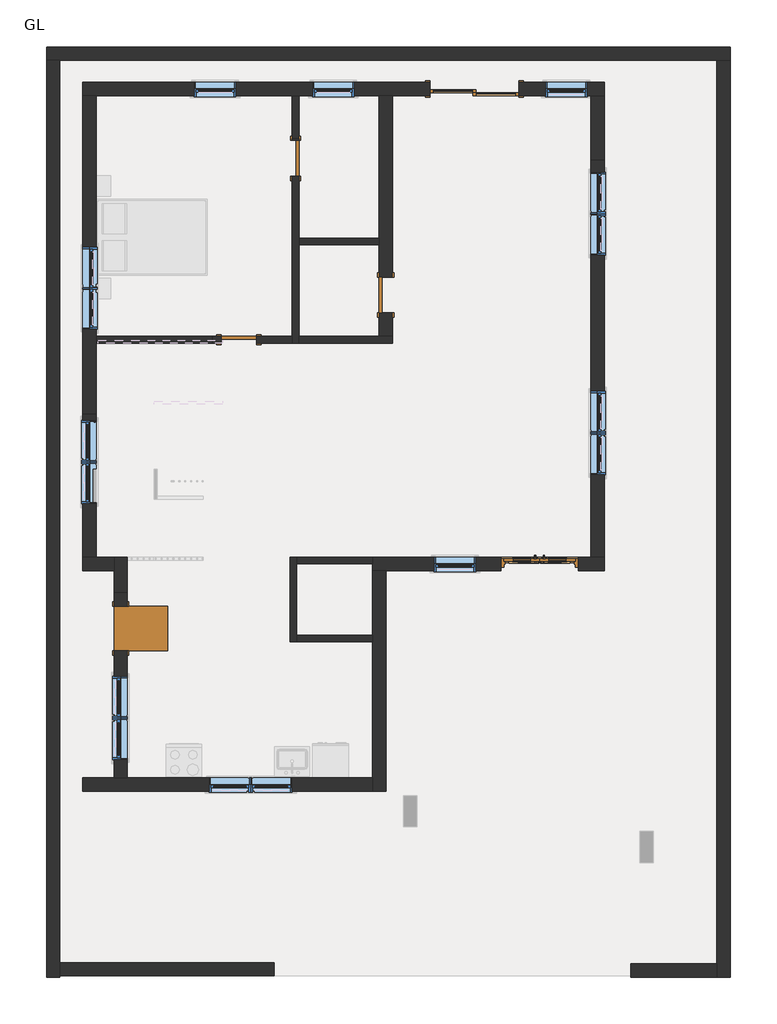
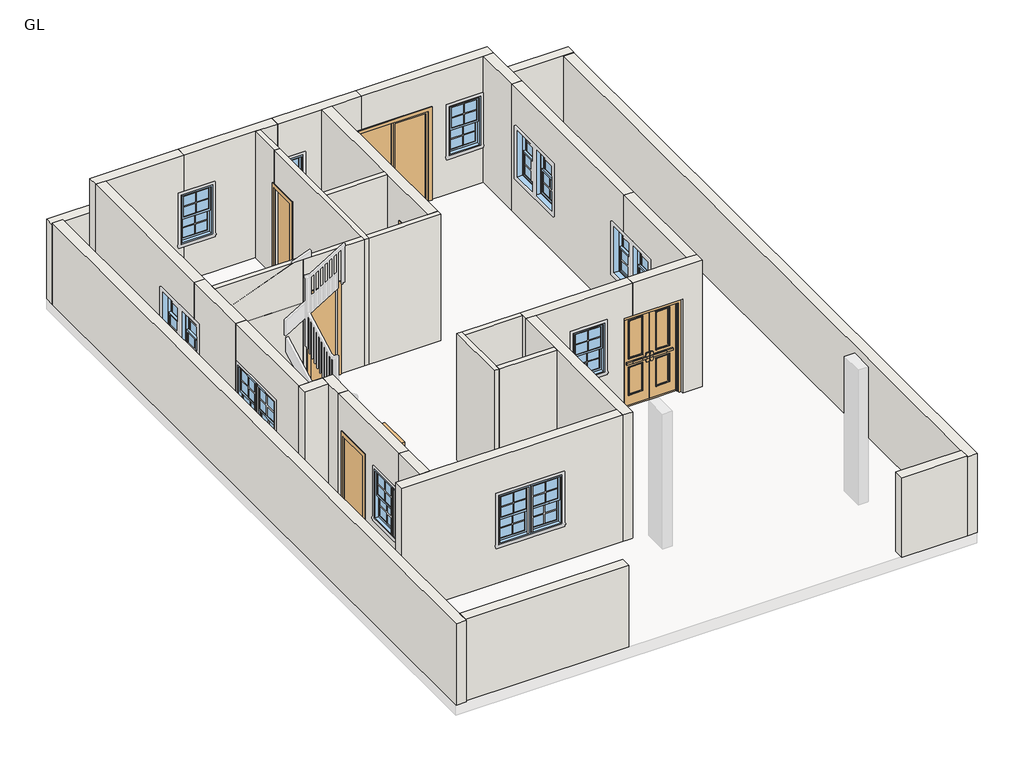
# One storey, part 1 of 3: 33 walls, 16 windows, 6 doors.
"""IFC4 building model written with IfcOpenShell, lengths in millimetres."""

from ifc_helpers import new_model, si_unit, frame, origin, origin_with_axes, place, context, project, spatial, polyline, outline, extrude, faceted_brep, transform, mapped, element, save
from components import door_238c678e, door_exterior_double_two_lite_door_exterior_double_two_lite_a6b01c7a, door_exterior_double_two_lite_door_exterior_double_two_lite_31e28e64, door_exterior_double_two_lite_door_exterior_double_two_lite_4a402bc0, single_flush_2_x_7_f433b8c7, door_0bf9f8da, door_0d3b4037, window_fc4bf0c6

model = new_model("IFC4")

# Units and contexts
model_context = context("Model", 3, world=origin())
ifc_project = project(units=[si_unit("LENGTHUNIT", "METRE", prefix="MILLI")], contexts=[model_context])

# Site, building, storey
site = spatial("IfcSite", under=ifc_project)
building = spatial("IfcBuilding", under=site)
storey = spatial("IfcBuildingStorey", under=building, Name="GL", Elevation=0.0)

# Doors
placement = place(None, origin())
door_shape = door_238c678e(model_context)
element("IfcDoor", 1, ObjectType="Door-Double-Sliding : 60\" x 84\"", at=placement, inside=storey, context=model_context, shape_type="MappedRepresentation", body=[
    mapped(door_shape, transform((-15781.8310804, 12791.3223147, 0.0), x_axis=(-1.0, 0.0, 0.0), y_axis=(0.0, -1.0, 0.0), z_axis=(0.0, 0.0, 1.0))),
])
door_exterior_double_two_lite_door_exterior_double_two_lite_shape = door_exterior_double_two_lite_door_exterior_double_two_lite_a6b01c7a(model_context)
door_exterior_double_two_lite_door_exterior_double_two_lite_2_shape = door_exterior_double_two_lite_door_exterior_double_two_lite_31e28e64(model_context)
door_exterior_double_two_lite_door_exterior_double_two_lite_3_shape = door_exterior_double_two_lite_door_exterior_double_two_lite_4a402bc0(model_context)
element("IfcDoor", 2, ObjectType="Door-Exterior-Double-Two_Lite : Door-Exterior-Double-Two_Lite", at=placement, inside=storey, context=model_context, shape_type="MappedRepresentation", body=[
    mapped(door_exterior_double_two_lite_door_exterior_double_two_lite_shape, transform((-14665.6751671, 4542.6723646, 0.0), x_axis=(1.0, 0.0, 0.0), y_axis=(0.0, 1.0, 0.0), z_axis=(0.0, 0.0, 1.0))),
    mapped(door_exterior_double_two_lite_door_exterior_double_two_lite_2_shape, transform((-14665.6751671, 4542.6723646, 0.0), x_axis=(1.0, 0.0, 0.0), y_axis=(0.0, 1.0, 0.0), z_axis=(0.0, 0.0, 1.0))),
    mapped(door_exterior_double_two_lite_door_exterior_double_two_lite_3_shape, transform((-14665.6751671, 4542.6723646, 0.0), x_axis=(1.0, 0.0, 0.0), y_axis=(0.0, 1.0, 0.0), z_axis=(0.0, 0.0, 1.0))),
])
single_flush_2_x_7_shape = single_flush_2_x_7_f433b8c7(model_context)
element("IfcDoor", 3, ObjectType="Single-Flush : 2' x 7'", at=placement, inside=storey, context=model_context, shape_type="MappedRepresentation", body=[
    mapped(single_flush_2_x_7_shape, transform((-21828.4750314, 3444.1223646, 0.0), x_axis=(0.0, 1.0, 0.0), y_axis=(-1.0, 0.0, 0.0), z_axis=(0.0, 0.0, 1.0))),
])
door_2_shape = door_0bf9f8da(model_context)
element("IfcDoor", 4, ObjectType="Single-Flush : 24\" x 84\"", at=placement, inside=storey, context=model_context, shape_type="MappedRepresentation", body=[
    mapped(door_2_shape, transform((-18837.6250314, 11478.1423646, 0.0), x_axis=(0.0, 1.0, 0.0), y_axis=(-1.0, 0.0, 0.0), z_axis=(0.0, 0.0, 1.0))),
])
element("IfcDoor", 5, ObjectType="Single-Flush : 24\" x 84\"", at=placement, inside=storey, context=model_context, shape_type="MappedRepresentation", body=[
    mapped(door_2_shape, transform((-19809.1750314, 8378.0723646, 0.0), x_axis=(-1.0, 0.0, 0.0), y_axis=(0.0, -1.0, 0.0), z_axis=(0.0, 0.0, 1.0))),
])
door_3_shape = door_0d3b4037(model_context)
element("IfcDoor", 6, ObjectType="Single-Flush : 24\" x 84\"", at=placement, inside=storey, context=model_context, shape_type="MappedRepresentation", body=[
    mapped(door_3_shape, transform((-17294.5750314, 9140.0723646, 0.0), x_axis=(0.0, 1.0, 0.0), y_axis=(-1.0, 0.0, 0.0), z_axis=(0.0, 0.0, 1.0))),
])

# Walls
element("IfcWall", 7, ObjectType="Generic - 4.5\"", at=placement, inside=storey, context=model_context, shape_type="SweptSolid", body=[
    extrude(outline(polyline([(-18894.7750314, 11808.3423646), (-18894.7750314, 12550.0223147), (-18780.4750314, 12550.0223147), (-18780.4750314, 11808.3423646), (-18894.7750314, 11808.3423646)])), origin_with_axes(), (0.0, 0.0, 1.0), 2997.2),
])
element("IfcWall", 8, ObjectType="Generic - 4.5\"", at=placement, inside=storey, context=model_context, shape_type="Brep", body=[
    faceted_brep([(-18894.7750314, 11808.3423646, 0.0), (-18894.7750314, 11782.9423646, 0.0), (-18894.7750314, 11782.9423646, 2133.6), (-18894.7750314, 11173.3423646, 2133.6), (-18894.7750314, 11173.3423646, 0.0), (-18894.7750314, 8435.2223646, 0.0), (-18894.7750314, 8320.9223646, 0.0), (-18894.7750314, 8320.9223646, 2997.2), (-18894.7750314, 8435.2223646, 2997.2), (-18894.7750314, 11808.3423646, 2997.2), (-18780.4750314, 11782.9423646, 2133.6), (-18780.4750314, 11782.9423646, 0.0), (-18780.4750314, 11808.3423646, 0.0), (-18780.4750314, 11808.3423646, 2997.2), (-18780.4750314, 10111.6223646, 2997.2), (-18780.4750314, 9997.3223646, 2997.2), (-18780.4750314, 8435.2223646, 2997.2), (-18780.4750314, 8320.9223646, 2997.2), (-18780.4750314, 8320.9223646, 0.0), (-18780.4750314, 8435.2223646, 0.0), (-18780.4750314, 9997.3223646, 0.0), (-18780.4750314, 10111.6223646, 0.0), (-18780.4750314, 11173.3423646, 0.0), (-18780.4750314, 11173.3423646, 2133.6)], [[[0, 1, 2, 3, 4, 5, 6, 7, 8, 9]], [[10, 11, 12, 13, 14, 15, 16, 17, 18, 19, 20, 21, 22, 23]], [[12, 11, 1, 0]], [[22, 21, 20, 19, 18, 6, 5, 4]], [[0, 9, 13, 12]], [[7, 6, 18, 17]], [[2, 1, 11, 10]], [[3, 2, 10, 23]], [[4, 3, 23, 22]], [[9, 8, 7, 17, 16, 15, 14, 13]]]),
])
element("IfcWall", 9, ObjectType="Generic - 4.5\"", at=placement, inside=storey, context=model_context, shape_type="Brep", body=[
    faceted_brep([(-18780.4750314, 8320.9223646, 0.0), (-17180.2750314, 8320.9223646, 0.0), (-17180.2750314, 8320.9223646, 2997.2), (-18780.4750314, 8320.9223646, 2997.2), (-18780.4750314, 8435.2223646, 0.0), (-18780.4750314, 8435.2223646, 2997.2), (-17408.8750314, 8435.2223646, 2997.2), (-17180.2750314, 8435.2223646, 2997.2), (-17180.2750314, 8435.2223646, 0.0), (-17408.8750314, 8435.2223646, 0.0)], [[[0, 1, 2, 3]], [[4, 5, 6, 7, 8, 9]], [[1, 0, 4, 9, 8]], [[0, 3, 5, 4]], [[2, 1, 8, 7]], [[3, 2, 7, 6, 5]]]),
])
element("IfcWall", 10, ObjectType="Generic - 4.5\"", at=placement, inside=storey, context=model_context, shape_type="SweptSolid", body=[
    extrude(outline(polyline([(0.0, -20266.3750314), (0.0, -20113.9750314), (2133.6, -20113.9750314), (2133.6, -19504.3750314), (0.0, -19504.3750314), (0.0, -18894.7750314), (2997.2, -18894.7750314), (2997.2, -20266.3750314), (0.0, -20266.3750314)])), frame((0.0, 8320.9223646, 0.0), z_axis=(0.0, 1.0, 0.0), x_axis=(0.0, 0.0, 1.0)), (0.0, 0.0, 1.0), 114.3),
])
element("IfcWall", 11, ObjectType="Generic - 4.5\"", at=placement, inside=storey, context=model_context, shape_type="SweptSolid", body=[
    extrude(outline(polyline([(-20266.3750314, 8320.9223646), (-22247.5752061, 8320.9223646), (-22247.5752061, 8435.2223646), (-20266.3750314, 8435.2223646), (-20266.3750314, 8320.9223646)])), origin_with_axes(), (0.0, 0.0, 1.0), 2997.2),
])
element("IfcWall", 12, ObjectType="Generic - 4.5\"", at=placement, inside=storey, context=model_context, shape_type="SweptSolid", body=[
    extrude(outline(polyline([(-17408.8750314, 9997.3223646), (-18780.4750314, 9997.3223646), (-18780.4750314, 10111.6223646), (-17408.8750314, 10111.6223646), (-17408.8750314, 9997.3223646)])), origin_with_axes(), (0.0, 0.0, 1.0), 2997.2),
])
element("IfcWall", 13, ObjectType="Generic - 4.5\"", at=placement, inside=storey, context=model_context, shape_type="Brep", body=[
    faceted_brep([(-18932.8750314, 4663.3223646, 0.0), (-18932.8750314, 3215.5223646, 0.0), (-18932.8750314, 3215.5223646, 2997.2), (-18932.8750314, 4663.3223646, 2997.2), (-18818.5750314, 4663.3223646, 0.0), (-18818.5750314, 4663.3223646, 2997.2), (-18818.5750314, 4549.0223646, 2997.2), (-18818.5750314, 3329.8223646, 2997.2), (-18818.5750314, 3215.5223646, 2997.2), (-18818.5750314, 3215.5223646, 0.0), (-18818.5750314, 3329.8223646, 0.0), (-18818.5750314, 4549.0223646, 0.0)], [[[0, 1, 2, 3]], [[4, 5, 6, 7, 8, 9, 10, 11]], [[1, 0, 4, 11, 10, 9]], [[2, 1, 9, 8]], [[0, 3, 5, 4]], [[3, 2, 8, 7, 6, 5]]]),
])
element("IfcWall", 14, ObjectType="Generic - 4.5\"", at=placement, inside=storey, context=model_context, shape_type="SweptSolid", body=[
    extrude(outline(polyline([(-17523.1750314, 3215.5223646), (-18818.5750314, 3215.5223646), (-18818.5750314, 3329.8223646), (-17523.1750314, 3329.8223646), (-17523.1750314, 3215.5223646)])), origin_with_axes(), (0.0, 0.0, 1.0), 2997.2),
])
element("IfcWall", 15, ObjectType="Generic - 4.5\"", at=placement, inside=storey, context=model_context, shape_type="SweptSolid", body=[
    extrude(outline(polyline([(-17523.1750314, 4549.0223646), (-18818.5750314, 4549.0223646), (-18818.5750314, 4663.3223646), (-17523.1750314, 4663.3223646), (-17523.1750314, 4549.0223646)])), origin_with_axes(), (0.0, 0.0, 1.0), 2997.2),
])
element("IfcWall", 16, ObjectType="Generic - 9\" 2", at=placement, inside=storey, context=model_context, shape_type="Brep", body=[
    faceted_brep([(-11408.7437595, 13378.6077942, 0.0), (-23096.6616791, 13378.6077942, 0.0), (-23096.6616791, 13378.6077942, 1886.4124862), (-11408.7437595, 13378.6077942, 1886.4124862), (-11408.7437595, 13150.0077942, 0.0), (-11408.7437595, 13150.0077942, 1876.4849166), (-11408.7437595, 13150.0077942, 1886.4124862), (-23096.6616791, 13150.0077942, 1886.4124862), (-23096.6616791, 13150.0077942, 0.0), (-22868.0616791, 13150.0077942, 0.0), (-11637.3437595, 13150.0077942, 0.0)], [[[0, 1, 2, 3]], [[4, 5, 6, 7, 8, 9, 10]], [[1, 0, 4, 10, 9, 8]], [[3, 2, 7, 6]], [[2, 1, 8, 7]], [[0, 3, 6, 5, 4]]]),
])
element("IfcWall", 17, ObjectType="Generic - 9\" 2", at=placement, inside=storey, context=model_context, shape_type="Brep", body=[
    faceted_brep([(-23096.6616791, 13150.0077942, 0.0), (-23096.6616791, -2518.5276354, 0.0), (-23096.6616791, -2518.5276354, 1930.400068), (-23096.6616791, 13150.0077942, 1930.400068), (-23096.6616791, 13150.0077942, 1886.4124862), (-22868.0616791, 13150.0077942, 0.0), (-22868.0616791, 13150.0077942, 1930.400068), (-22868.0616791, -2518.5276354, 1930.400068), (-22868.0616791, -2518.5276354, 0.0)], [[[0, 1, 2, 3, 4]], [[5, 6, 7, 8]], [[1, 0, 5, 8]], [[2, 1, 8, 7]], [[3, 2, 7, 6]], [[0, 4, 3, 6, 5]]]),
])
element("IfcWall", 18, ObjectType="Generic - 9\" 2", at=placement, inside=storey, context=model_context, shape_type="SweptSolid", body=[
    extrude(outline(polyline([(-19208.5067292, -2492.7076157), (-22866.1067292, -2492.7076157), (-22866.1067292, -2264.1076157), (-19208.5067292, -2264.1076157), (-19208.5067292, -2492.7076157)])), origin_with_axes(), (0.0, 0.0, 1.0), 1937.5226212),
])
element("IfcWall", 19, ObjectType="Generic - 9\" 2", at=placement, inside=storey, context=model_context, shape_type="Brep", body=[
    faceted_brep([(-11637.3437595, 13150.0077942, 0.0), (-11637.3437595, -2286.8422058, 0.0), (-11637.3437595, -2515.4422058, 0.0), (-11637.3437595, -2515.4422058, 1876.4849166), (-11637.3437595, 13150.0077942, 1876.4849166), (-11408.7437595, 13150.0077942, 0.0), (-11408.7437595, 13150.0077942, 1876.4849166), (-11408.7437595, -2515.4422058, 1876.4849166), (-11408.7437595, -2515.4422058, 0.0)], [[[0, 1, 2, 3, 4]], [[5, 6, 7, 8]], [[2, 1, 0, 5, 8]], [[4, 3, 7, 6]], [[0, 4, 6, 5]], [[3, 2, 8, 7]]]),
])
element("IfcWall", 20, ObjectType="Generic - 9\" 2", at=placement, inside=storey, context=model_context, shape_type="Brep", body=[
    faceted_brep([(-11637.3437595, -2286.8422058, 0.0), (-13103.5750314, -2286.8422058, 0.0), (-13103.5750314, -2286.8422058, 1892.5418489), (-11637.3437595, -2286.8422058, 1892.5418489), (-11637.3437595, -2515.4422058, 0.0), (-11637.3437595, -2515.4422058, 1876.4849166), (-11637.3437595, -2515.4422058, 1892.5418489), (-13103.5750314, -2515.4422058, 1892.5418489), (-13103.5750314, -2515.4422058, 0.0)], [[[0, 1, 2, 3]], [[4, 5, 6, 7, 8]], [[1, 0, 4, 8]], [[2, 1, 8, 7]], [[3, 2, 7, 6]], [[0, 3, 6, 5, 4]]]),
])
element("IfcWall", 21, ObjectType="Generic -9\"Brick 2", at=placement, inside=storey, context=model_context, shape_type="Brep", body=[
    faceted_brep([(-22476.1750314, 12550.0223646, 0.0), (-22247.5750314, 12550.0223646, 0.0), (-20494.9750314, 12550.0223646, 0.0), (-20494.9750314, 12550.0223646, 914.4), (-20571.1750314, 12550.0223646, 914.4), (-20571.1750314, 12550.0223646, 2082.8), (-20494.9750314, 12550.0223646, 2082.8), (-20494.9750314, 12550.0223646, 2997.2), (-22247.5750314, 12550.0223646, 2997.2), (-22476.1752061, 12550.0223646, 2997.2), (-20494.9750314, 12778.6223646, 0.0), (-22476.1750314, 12778.6223646, 0.0), (-22476.1750314, 12778.6223646, 2997.2), (-20494.9750314, 12778.6223646, 2997.2), (-20494.9750314, 12778.6223646, 2082.8), (-20571.1750314, 12778.6223646, 2082.8), (-20571.1750314, 12778.6223646, 914.4), (-20494.9750314, 12778.6223646, 914.4)], [[[0, 1, 2, 3, 4, 5, 6, 7, 8, 9]], [[10, 11, 12, 13, 14, 15, 16, 17]], [[2, 1, 0, 11, 10]], [[2, 10, 17, 3]], [[13, 7, 6, 14]], [[0, 9, 12, 11]], [[16, 4, 3, 17]], [[4, 16, 15, 5]], [[5, 15, 14, 6]], [[9, 8, 7, 13, 12]]]),
])
element("IfcWall", 22, ObjectType="Generic -9\"Brick 2", at=placement, inside=storey, context=model_context, shape_type="Brep", body=[
    faceted_brep([(-20494.9750314, 12550.0223147, 0.0), (-18894.7750314, 12550.0223147, 0.0), (-18780.4750314, 12550.0223147, 0.0), (-18397.0494379, 12550.0223147, 0.0), (-18397.0494379, 12550.0223147, 914.4), (-18549.4494379, 12550.0223147, 914.4), (-18549.4494379, 12550.0223147, 2082.8), (-18397.0494379, 12550.0223147, 2082.8), (-18397.0494379, 12550.0223147, 2997.2), (-18780.4750314, 12550.0223147, 2997.2), (-18894.7750314, 12550.0223147, 2997.2), (-20494.9750314, 12550.0223147, 2997.2), (-20494.9750314, 12550.0223147, 2082.8), (-19859.9750314, 12550.0223147, 2082.8), (-19859.9750314, 12550.0223147, 914.4), (-20494.9750314, 12550.0223147, 914.4), (-18397.0494379, 12778.6223147, 0.0), (-20494.9750314, 12778.6223147, 0.0), (-20494.9750314, 12778.6223147, 914.4), (-19859.9750314, 12778.6223147, 914.4), (-19859.9750314, 12778.6223147, 2082.8), (-20494.9750314, 12778.6223147, 2082.8), (-20494.9750314, 12778.6223147, 2997.2), (-18397.0494379, 12778.6223147, 2997.2), (-18397.0494379, 12778.6223147, 2082.8), (-18549.4494379, 12778.6223147, 2082.8), (-18549.4494379, 12778.6223147, 914.4), (-18397.0494379, 12778.6223147, 914.4)], [[[0, 1, 2, 3, 4, 5, 6, 7, 8, 9, 10, 11, 12, 13, 14, 15]], [[16, 17, 18, 19, 20, 21, 22, 23, 24, 25, 26, 27]], [[3, 2, 1, 0, 17, 16]], [[3, 16, 27, 4]], [[23, 8, 7, 24]], [[17, 0, 15, 18]], [[12, 11, 22, 21]], [[13, 20, 19, 14]], [[14, 19, 18, 15]], [[20, 13, 12, 21]], [[26, 5, 4, 27]], [[5, 26, 25, 6]], [[6, 25, 24, 7]], [[11, 10, 9, 8, 23, 22]]]),
])
element("IfcWall", 23, ObjectType="Generic -9\"Brick 2", at=placement, inside=storey, context=model_context, shape_type="Brep", body=[
    faceted_brep([(-18397.0494379, 12550.0223147, 914.4), (-18397.0494379, 12550.0223147, 0.0), (-17408.8750314, 12550.0223147, 0.0), (-17180.2750314, 12550.0223147, 0.0), (-16543.8310804, 12550.0223147, 0.0), (-16543.8310804, 12550.0223147, 2133.6), (-16518.4310804, 12550.0223147, 2133.6), (-16518.4310804, 12550.0223147, 2997.2), (-17180.2750314, 12550.0223147, 2997.2), (-17408.8750314, 12550.0223147, 2997.2), (-18397.0494379, 12550.0223147, 2997.2), (-18397.0494379, 12550.0223147, 2082.8), (-17838.2494379, 12550.0223147, 2082.8), (-17838.2494379, 12550.0223147, 914.4), (-18397.0494379, 12778.6223147, 0.0), (-18397.0494379, 12778.6223147, 914.4), (-17838.2494379, 12778.6223147, 914.4), (-17838.2494379, 12778.6223147, 2082.8), (-18397.0494379, 12778.6223147, 2082.8), (-18397.0494379, 12778.6223147, 2997.2), (-16518.4310804, 12778.6223147, 2997.2), (-16518.4310804, 12778.6223147, 2133.6), (-16543.8310804, 12778.6223147, 2133.6), (-16543.8310804, 12778.6223147, 0.0)], [[[0, 1, 2, 3, 4, 5, 6, 7, 8, 9, 10, 11, 12, 13]], [[14, 15, 16, 17, 18, 19, 20, 21, 22, 23]], [[1, 14, 23, 4, 3, 2]], [[20, 7, 6, 21]], [[14, 1, 0, 15]], [[11, 10, 19, 18]], [[12, 17, 16, 13]], [[13, 16, 15, 0]], [[17, 12, 11, 18]], [[22, 5, 4, 23]], [[5, 22, 21, 6]], [[10, 9, 8, 7, 20, 19]]]),
])
element("IfcWall", 24, ObjectType="Generic -9\"Brick 2", at=placement, inside=storey, context=model_context, shape_type="Brep", body=[
    faceted_brep([(-13560.7750314, 12550.0223147, 0.0), (-13560.7750314, 12550.0223147, 2997.2), (-13789.3750314, 12550.0223147, 2997.2), (-16518.4310804, 12550.0223147, 2997.2), (-16518.4310804, 12550.0223147, 2133.6), (-15019.8310804, 12550.0223147, 2133.6), (-15019.8310804, 12550.0223147, 0.0), (-13789.3750314, 12550.0223147, 0.0), (-13852.8750314, 12550.0223147, 2082.8), (-13852.8750314, 12550.0223147, 914.4), (-14564.0750314, 12550.0223147, 914.4), (-14564.0750314, 12550.0223147, 2082.8), (-13560.7750314, 12778.6223147, 2997.2), (-13560.7750314, 12778.6223147, 0.0), (-15019.8310804, 12778.6223147, 0.0), (-15019.8310804, 12778.6223147, 2133.6), (-16518.4310804, 12778.6223147, 2133.6), (-16518.4310804, 12778.6223147, 2997.2), (-13852.8750314, 12778.6223147, 2082.8), (-14564.0750314, 12778.6223147, 2082.8), (-14564.0750314, 12778.6223147, 914.4), (-13852.8750314, 12778.6223147, 914.4)], [[[0, 1, 2, 3, 4, 5, 6, 7], [8, 9, 10, 11]], [[12, 13, 14, 15, 16, 17], [18, 19, 20, 21]], [[13, 0, 7, 6, 14]], [[3, 17, 16, 4]], [[1, 0, 13, 12]], [[9, 8, 18, 21]], [[10, 9, 21, 20]], [[11, 10, 20, 19]], [[8, 11, 19, 18]], [[5, 15, 14, 6]], [[15, 5, 4, 16]], [[3, 2, 1, 12, 17]]]),
])
element("IfcWall", 25, ObjectType="Generic -9\"Brick 2", at=placement, inside=storey, context=model_context, shape_type="SweptSolid", body=[
    extrude(outline(polyline([(-13789.3750314, 11447.1098201), (-13789.3750314, 12550.0223147), (-13560.7750314, 12550.0223147), (-13560.7750314, 11447.1098201), (-13789.3750314, 11447.1098201)])), origin_with_axes(), (0.0, 0.0, 1.0), 2997.2),
])
element("IfcWall", 26, ObjectType="Generic -9\"Brick 2", at=placement, inside=storey, context=model_context, shape_type="SweptSolid", body=[
    extrude(outline(polyline([(11447.1098201, 0.0), (7101.7223647, 0.0), (7101.7223647, 914.4), (7495.4223646, 914.4), (7495.4223646, 2082.8), (7101.7223647, 2082.8), (7101.7223647, 2997.2), (11447.1098201, 2997.2), (11447.1098201, 0.0)]), holes=[polyline([(11243.9098201, 914.4), (11243.9098201, 2082.8), (9821.5098201, 2082.8), (9821.5098201, 914.4), (11243.9098201, 914.4)])]), frame((-13789.3750314, 0.0, 0.0), z_axis=(1.0, 0.0, 0.0), x_axis=(0.0, 1.0, 0.0)), (0.0, 0.0, 1.0), 228.6),
])
element("IfcWall", 27, ObjectType="Generic -9\"Brick 2", at=placement, inside=storey, context=model_context, shape_type="SweptSolid", body=[
    extrude(outline(polyline([(7101.7223647, 0.0), (4663.3223646, 0.0), (4663.3223646, 2997.2), (7101.7223647, 2997.2), (7101.7223647, 2082.8), (6073.0223646, 2082.8), (6073.0223646, 914.4), (7101.7223647, 914.4), (7101.7223647, 0.0)])), frame((-13789.3750314, 0.0, 0.0), z_axis=(1.0, 0.0, 0.0), x_axis=(0.0, 1.0, 0.0)), (0.0, 0.0, 1.0), 228.6),
])
element("IfcWall", 28, ObjectType="Generic -9\"Brick 2", at=placement, inside=storey, context=model_context, shape_type="Brep", body=[
    faceted_brep([(-13560.7750314, 4434.7223646, 0.0), (-13560.7750314, 4434.7223646, 2997.2), (-15122.8751671, 4434.7223646, 2997.2), (-15122.8751671, 4434.7223646, 2235.2), (-14005.2751671, 4434.7223646, 2235.2), (-14005.2751671, 4434.7223646, 0.0), (-13560.7750314, 4663.3223646, 2997.2), (-13560.7750314, 4663.3223646, 0.0), (-13789.3750314, 4663.3223646, 0.0), (-14005.2751671, 4663.3223646, 0.0), (-14005.2751671, 4663.3223646, 2235.2), (-15122.8751671, 4663.3223646, 2235.2), (-15122.8751671, 4663.3223646, 2997.2), (-13789.3750314, 4663.3223646, 2997.2)], [[[0, 1, 2, 3, 4, 5]], [[6, 7, 8, 9, 10, 11, 12, 13]], [[7, 0, 5, 9, 8]], [[2, 12, 11, 3]], [[1, 0, 7, 6]], [[4, 10, 9, 5]], [[10, 4, 3, 11]], [[2, 1, 6, 13, 12]]]),
])
element("IfcWall", 29, ObjectType="Generic -9\"Brick 2", at=placement, inside=storey, context=model_context, shape_type="Brep", body=[
    faceted_brep([(-17523.1750314, 4663.3223722, 0.0), (-17523.1750314, 4663.3223722, 2997.2), (-15122.8751671, 4663.3223722, 2997.2), (-15122.8751671, 4663.3223722, 2235.2), (-15326.0751671, 4663.3223722, 2235.2), (-15326.0751671, 4663.3223722, 0.0), (-15757.8750314, 4663.3223722, 2290.2004923), (-16469.0750314, 4663.3223722, 2290.2004923), (-16469.0750314, 4663.3223722, 1121.8004923), (-15757.8750314, 4663.3223722, 1121.8004923), (-17523.1750314, 4434.7223722, 2997.2), (-17523.1750314, 4434.7223722, 0.0), (-17294.5750314, 4434.7223722, 0.0), (-15326.0751671, 4434.7223722, 0.0), (-15326.0751671, 4434.7223722, 2235.2), (-15122.8751671, 4434.7223722, 2235.2), (-15122.8751671, 4434.7223722, 2997.2), (-17294.5750314, 4434.7223722, 2997.2), (-15757.8750314, 4434.7223722, 2290.2004923), (-15757.8750314, 4434.7223722, 1121.8004923), (-16469.0750314, 4434.7223722, 1121.8004923), (-16469.0750314, 4434.7223722, 2290.2004923), (-17523.1750314, 4549.0223646, 0.0), (-17523.1750314, 4549.0223646, 2997.2)], [[[0, 1, 2, 3, 4, 5], [6, 7, 8, 9]], [[10, 11, 12, 13, 14, 15, 16, 17], [18, 19, 20, 21]], [[11, 22, 0, 5, 13, 12]], [[2, 16, 15, 3]], [[1, 0, 22, 11, 10, 23]], [[14, 4, 3, 15]], [[4, 14, 13, 5]], [[2, 1, 23, 10, 17, 16]], [[19, 18, 6, 9]], [[20, 19, 9, 8]], [[21, 20, 8, 7]], [[18, 21, 7, 6]]]),
])
element("IfcWall", 30, ObjectType="Generic -9\"Brick 2", at=placement, inside=storey, context=model_context, shape_type="Brep", body=[
    faceted_brep([(-17523.1750314, 4434.7223722, 0.0), (-17523.1750314, 3329.8223646, 0.0), (-17523.1750314, 3215.5223646, 0.0), (-17523.1750314, 891.4223646, 0.0), (-17523.1750314, 662.8223646, 0.0), (-17523.1750314, 662.8223646, 2997.2), (-17523.1750314, 891.4223646, 2997.2), (-17523.1750314, 3215.5223646, 2997.2), (-17523.1750314, 3329.8223646, 2997.2), (-17523.1750314, 4434.7223722, 2997.2), (-17294.5750314, 4434.7223722, 0.0), (-17294.5750314, 4434.7223722, 2997.2), (-17294.5750314, 662.8223646, 2997.2), (-17294.5750314, 662.8223646, 0.0)], [[[0, 1, 2, 3, 4, 5, 6, 7, 8, 9]], [[10, 11, 12, 13]], [[4, 3, 2, 1, 0, 10, 13]], [[0, 9, 11, 10]], [[5, 4, 13, 12]], [[9, 8, 7, 6, 5, 12, 11]]]),
])
element("IfcWall", 31, ObjectType="Generic -9\"Brick 2", at=placement, inside=storey, context=model_context, shape_type="Brep", body=[
    faceted_brep([(-17523.1750314, 891.4223646, 0.0), (-21714.1750314, 891.4223646, 0.0), (-21942.7750314, 891.4223646, 0.0), (-22476.1750314, 891.4223646, 0.0), (-22476.1750314, 891.4223646, 2997.2), (-21942.7750314, 891.4223646, 2997.2), (-21714.1750314, 891.4223646, 2997.2), (-17523.1750314, 891.4223646, 2997.2), (-18894.6931686, 891.4223646, 2082.8), (-20317.0931686, 891.4223646, 2082.8), (-20317.0931686, 891.4223646, 914.4), (-18894.6931686, 891.4223646, 914.4), (-22476.1750314, 662.8223646, 0.0), (-17523.1750314, 662.8223646, 0.0), (-17523.1750314, 662.8223646, 2997.2), (-22476.1750314, 662.8223646, 2997.2), (-20317.0931686, 662.8223646, 2082.8), (-18894.6931686, 662.8223646, 2082.8), (-18894.6931686, 662.8223646, 914.4), (-20317.0931686, 662.8223646, 914.4)], [[[0, 1, 2, 3, 4, 5, 6, 7], [8, 9, 10, 11]], [[12, 13, 14, 15], [16, 17, 18, 19]], [[3, 2, 1, 0, 13, 12]], [[4, 3, 12, 15]], [[0, 7, 14, 13]], [[16, 9, 8, 17]], [[18, 11, 10, 19]], [[18, 17, 8, 11]], [[19, 10, 9, 16]], [[7, 6, 5, 4, 15, 14]]]),
])
element("IfcWall", 32, ObjectType="Generic -9\"Brick 2", at=placement, inside=storey, context=model_context, shape_type="SweptSolid", body=[
    extrude(outline(polyline([(1710.5723646, 0.0), (891.4223646, 0.0), (891.4223646, 2997.2), (1710.5723646, 2997.2), (1710.5723646, 2082.8), (1202.5723646, 2082.8), (1202.5723646, 914.4), (1710.5723646, 914.4), (1710.5723646, 0.0)])), frame((-21942.7750314, 0.0, 0.0), z_axis=(1.0, 0.0, 0.0), x_axis=(0.0, 1.0, 0.0)), (0.0, 0.0, 1.0), 228.6),
])
element("IfcWall", 33, ObjectType="Generic -9\"Brick 2", at=placement, inside=storey, context=model_context, shape_type="SweptSolid", body=[
    extrude(outline(polyline([(4053.7223646, 0.0), (3825.1223646, 0.0), (3825.1223646, 2133.6), (3063.1223646, 2133.6), (3063.1223646, 0.0), (1710.5723646, 0.0), (1710.5723646, 914.4), (2624.9723646, 914.4), (2624.9723646, 2082.8), (1710.5723646, 2082.8), (1710.5723646, 2997.2), (4053.7223646, 2997.2), (4053.7223646, 0.0)])), frame((-21942.7750314, 0.0, 0.0), z_axis=(1.0, 0.0, 0.0), x_axis=(0.0, 1.0, 0.0)), (0.0, 0.0, 1.0), 228.6),
])
element("IfcWall", 34, ObjectType="Generic -9\"Brick 2", at=placement, inside=storey, context=model_context, shape_type="Brep", body=[
    faceted_brep([(-21714.1750314, 4053.7223646, 0.0), (-21714.1750314, 4663.3223646, 0.0), (-21714.1750314, 4663.3223646, 2997.2), (-21714.1750314, 4053.7223646, 2997.2), (-21942.7750314, 4053.7223646, 0.0), (-21942.7750314, 4053.7223646, 2997.2), (-21942.7750314, 4434.7223646, 2997.2), (-21942.7750314, 4663.3223646, 2997.2), (-21942.7750314, 4663.3223646, 0.0), (-21942.7750314, 4434.7223646, 0.0)], [[[0, 1, 2, 3]], [[4, 5, 6, 7, 8, 9]], [[1, 0, 4, 9, 8]], [[0, 3, 5, 4]], [[2, 1, 8, 7]], [[3, 2, 7, 6, 5]]]),
])
element("IfcWall", 35, ObjectType="Generic -9\"Brick 2", at=placement, inside=storey, context=model_context, shape_type="SweptSolid", body=[
    extrude(outline(polyline([(12550.0223646, 0.0), (8710.539033, 0.0), (8710.539033, 914.4), (9955.139033, 914.4), (9955.139033, 2082.8), (8710.539033, 2082.8), (8710.539033, 2997.2), (12550.0223646, 2997.2), (12550.0223646, 0.0)])), frame((-22476.1750314, 0.0, 0.0), z_axis=(1.0, 0.0, 0.0), x_axis=(0.0, 1.0, 0.0)), (0.0, 0.0, 1.0), 228.6),
])
element("IfcWall", 36, ObjectType="Generic -9\"Brick 2", at=placement, inside=storey, context=model_context, shape_type="Brep", body=[
    faceted_brep([(-22476.1752061, 8710.539033, 0.0), (-22476.1752061, 7101.7223643, 0.0), (-22476.1752061, 7101.7223643, 2997.2), (-22476.1752061, 8710.539033, 2997.2), (-22476.1752061, 8710.539033, 2082.8), (-22476.1752061, 8558.139033, 2082.8), (-22476.1752061, 8558.139033, 914.4), (-22476.1752061, 8710.539033, 914.4), (-22247.5752061, 7101.7223643, 0.0), (-22247.5752061, 8320.9223646, 0.0), (-22247.5752061, 8435.2223646, 0.0), (-22247.5752061, 8710.539033, 0.0), (-22247.5752061, 8710.539033, 914.4), (-22247.5752061, 8558.139033, 914.4), (-22247.5752061, 8558.139033, 2082.8), (-22247.5752061, 8710.539033, 2082.8), (-22247.5752061, 8710.539033, 2997.2), (-22247.5752061, 8435.2223646, 2997.2), (-22247.5752061, 8320.9223646, 2997.2), (-22247.5752061, 7101.7223643, 2997.2)], [[[0, 1, 2, 3, 4, 5, 6, 7]], [[8, 9, 10, 11, 12, 13, 14, 15, 16, 17, 18, 19]], [[1, 0, 11, 10, 9, 8]], [[2, 1, 8, 19]], [[11, 0, 7, 12]], [[3, 16, 15, 4]], [[6, 13, 12, 7]], [[13, 6, 5, 14]], [[14, 5, 4, 15]], [[3, 2, 19, 18, 17, 16]]]),
])
element("IfcWall", 37, ObjectType="Generic -9\"Brick 2", at=placement, inside=storey, context=model_context, shape_type="SweptSolid", body=[
    extrude(outline(polyline([(7101.7223643, 0.0), (4663.3223646, 0.0), (4663.3223646, 2997.2), (7101.7223643, 2997.2), (7101.7223643, 0.0)]), holes=[polyline([(5577.7223643, 914.4), (7000.1223643, 914.4), (7000.1223643, 2082.8), (5577.7223643, 2082.8), (5577.7223643, 914.4)])]), frame((-22476.1752061, 0.0, 0.0), z_axis=(1.0, 0.0, 0.0), x_axis=(0.0, 1.0, 0.0)), (0.0, 0.0, 1.0), 228.6),
])
element("IfcWall", 38, ObjectType="Generic -9\"Brick 2", at=placement, inside=storey, context=model_context, shape_type="Brep", body=[
    faceted_brep([(-22476.1752061, 4434.7223646, 0.0), (-21942.7750314, 4434.7223646, 0.0), (-21942.7750314, 4434.7223646, 2997.2), (-22476.1752061, 4434.7223646, 2997.2), (-22476.1752061, 4663.3223646, 0.0), (-22476.1752061, 4663.3223646, 2997.2), (-22247.5752061, 4663.3223646, 2997.2), (-21942.7750314, 4663.3223646, 2997.2), (-21942.7750314, 4663.3223646, 0.0), (-22247.5752061, 4663.3223646, 0.0), (-22476.1752061, 4549.0223646, 2997.2), (-21942.7750314, 4549.0223646, 2997.2)], [[[0, 1, 2, 3]], [[4, 5, 6, 7, 8, 9]], [[1, 0, 4, 9, 8]], [[0, 3, 10, 5, 4]], [[2, 1, 8, 7, 11]], [[3, 2, 11, 7, 6, 5, 10]]]),
])
element("IfcWall", 39, ObjectType="Generic -9\"Brick 2", at=placement, inside=storey, context=model_context, shape_type="Brep", body=[
    faceted_brep([(-17408.8750314, 12550.0223147, 0.0), (-17408.8750314, 10111.6223646, 0.0), (-17408.8750314, 9997.3223646, 0.0), (-17408.8750314, 9444.8723646, 0.0), (-17408.8750314, 9444.8723646, 2133.6), (-17408.8750314, 8835.2723646, 2133.6), (-17408.8750314, 8835.2723646, 0.0), (-17408.8750314, 8435.2223646, 0.0), (-17408.8750314, 8435.2223646, 2997.2), (-17408.8750314, 9997.3223646, 2997.2), (-17408.8750314, 10111.6223646, 2997.2), (-17408.8750314, 12550.0223147, 2997.2), (-17180.2750314, 9444.8723646, 2133.6), (-17180.2750314, 9444.8723646, 0.0), (-17180.2750314, 12550.0223147, 0.0), (-17180.2750314, 12550.0223147, 2997.2), (-17180.2750314, 8435.2223646, 2997.2), (-17180.2750314, 8435.2223646, 0.0), (-17180.2750314, 8835.2723646, 0.0), (-17180.2750314, 8835.2723646, 2133.6)], [[[0, 1, 2, 3, 4, 5, 6, 7, 8, 9, 10, 11]], [[12, 13, 14, 15, 16, 17, 18, 19]], [[18, 17, 7, 6]], [[14, 13, 3, 2, 1, 0]], [[0, 11, 15, 14]], [[8, 7, 17, 16]], [[4, 3, 13, 12]], [[5, 4, 12, 19]], [[6, 5, 19, 18]], [[11, 10, 9, 8, 16, 15]]]),
])

# Windows
window_shape = window_fc4bf0c6(model_context)
element("IfcWindow", 40, ObjectType="Window-Double-Hung : 28\" x 46\"", at=placement, inside=storey, context=model_context, shape_type="MappedRepresentation", body=[
    mapped(window_shape, transform((-20215.5750314, 12664.3223147, 0.0), x_axis=(-1.0, 0.0, 0.0), y_axis=(0.0, -1.0, 0.0), z_axis=(0.0, 0.0, 1.0))),
])
element("IfcWindow", 41, ObjectType="Window-Double-Hung : 28\" x 46\"", at=placement, inside=storey, context=model_context, shape_type="MappedRepresentation", body=[
    mapped(window_shape, transform((-14208.4750314, 12664.3223147, 0.0), x_axis=(-1.0, 0.0, 0.0), y_axis=(0.0, -1.0, 0.0), z_axis=(0.0, 0.0, 1.0))),
])
element("IfcWindow", 42, ObjectType="Window-Double-Hung : 28\" x 46\"", at=placement, inside=storey, context=model_context, shape_type="MappedRepresentation", body=[
    mapped(window_shape, transform((-13675.0750314, 10888.3098201, 0.0), x_axis=(0.0, -1.0, 0.0), y_axis=(1.0, 0.0, 0.0), z_axis=(0.0, 0.0, 1.0))),
])
element("IfcWindow", 43, ObjectType="Window-Double-Hung : 28\" x 46\"", at=placement, inside=storey, context=model_context, shape_type="MappedRepresentation", body=[
    mapped(window_shape, transform((-13675.0750314, 10177.1098201, 0.0), x_axis=(0.0, -1.0, 0.0), y_axis=(1.0, 0.0, 0.0), z_axis=(0.0, 0.0, 1.0))),
])
element("IfcWindow", 44, ObjectType="Window-Double-Hung : 28\" x 46\"", at=placement, inside=storey, context=model_context, shape_type="MappedRepresentation", body=[
    mapped(window_shape, transform((-13675.0750314, 7139.8223646, 0.0), x_axis=(0.0, -1.0, 0.0), y_axis=(1.0, 0.0, 0.0), z_axis=(0.0, 0.0, 1.0))),
])
element("IfcWindow", 45, ObjectType="Window-Double-Hung : 28\" x 46\"", at=placement, inside=storey, context=model_context, shape_type="MappedRepresentation", body=[
    mapped(window_shape, transform((-13675.0750314, 6428.6223646, 0.0), x_axis=(0.0, -1.0, 0.0), y_axis=(1.0, 0.0, 0.0), z_axis=(0.0, 0.0, 1.0))),
])
element("IfcWindow", 46, ObjectType="Window-Double-Hung : 28\" x 46\"", at=placement, inside=storey, context=model_context, shape_type="MappedRepresentation", body=[
    mapped(window_shape, transform((-19961.4931686, 777.1223646, 0.0), x_axis=(-1.0, 0.0, 0.0), y_axis=(0.0, -1.0, 0.0), z_axis=(0.0, 0.0, 1.0))),
])
element("IfcWindow", 47, ObjectType="Window-Double-Hung : 28\" x 46\"", at=placement, inside=storey, context=model_context, shape_type="MappedRepresentation", body=[
    mapped(window_shape, transform((-19250.2931686, 777.1223646, 0.0), x_axis=(-1.0, 0.0, 0.0), y_axis=(0.0, -1.0, 0.0), z_axis=(0.0, 0.0, 1.0))),
])
element("IfcWindow", 48, ObjectType="Window-Double-Hung : 28\" x 46\"", at=placement, inside=storey, context=model_context, shape_type="MappedRepresentation", body=[
    mapped(window_shape, transform((-21828.4750314, 2269.3723646, 0.0), x_axis=(0.0, 1.0, 0.0), y_axis=(-1.0, 0.0, 0.0), z_axis=(0.0, 0.0, 1.0))),
])
element("IfcWindow", 49, ObjectType="Window-Double-Hung : 28\" x 46\"", at=placement, inside=storey, context=model_context, shape_type="MappedRepresentation", body=[
    mapped(window_shape, transform((-21828.4750314, 1558.1723646, 0.0), x_axis=(0.0, 1.0, 0.0), y_axis=(-1.0, 0.0, 0.0), z_axis=(0.0, 0.0, 1.0))),
])
element("IfcWindow", 50, ObjectType="Window-Double-Hung : 28\" x 46\"", at=placement, inside=storey, context=model_context, shape_type="MappedRepresentation", body=[
    mapped(window_shape, transform((-22361.8752061, 6644.5223643, 0.0), x_axis=(0.0, 1.0, 0.0), y_axis=(-1.0, 0.0, 0.0), z_axis=(0.0, 0.0, 1.0))),
])
element("IfcWindow", 51, ObjectType="Window-Double-Hung : 28\" x 46\"", at=placement, inside=storey, context=model_context, shape_type="MappedRepresentation", body=[
    mapped(window_shape, transform((-22361.8752061, 5933.3223643, 0.0), x_axis=(0.0, 1.0, 0.0), y_axis=(-1.0, 0.0, 0.0), z_axis=(0.0, 0.0, 1.0))),
])
element("IfcWindow", 52, ObjectType="Window-Double-Hung : 28\" x 46\"", at=placement, inside=storey, context=model_context, shape_type="MappedRepresentation", body=[
    mapped(window_shape, transform((-22361.8750314, 9599.539033, 0.0), x_axis=(0.0, -1.0, 0.0), y_axis=(1.0, 0.0, 0.0), z_axis=(0.0, 0.0, 1.0))),
])
element("IfcWindow", 53, ObjectType="Window-Double-Hung : 28\" x 46\"", at=placement, inside=storey, context=model_context, shape_type="MappedRepresentation", body=[
    mapped(window_shape, transform((-22361.8750314, 8913.739033, 0.0), x_axis=(0.0, -1.0, 0.0), y_axis=(1.0, 0.0, 0.0), z_axis=(0.0, 0.0, 1.0))),
])
element("IfcWindow", 54, ObjectType="Window-Double-Hung : 28\" x 46\"", at=placement, inside=storey, context=model_context, shape_type="MappedRepresentation", body=[
    mapped(window_shape, transform((-18193.8494379, 12664.3223147, 0.0), x_axis=(-1.0, 0.0, 0.0), y_axis=(0.0, -1.0, 0.0), z_axis=(0.0, 0.0, 1.0))),
])
element("IfcWindow", 55, ObjectType="Window-Double-Hung : 28\" x 46\"", at=placement, inside=storey, context=model_context, shape_type="MappedRepresentation", body=[
    mapped(window_shape, transform((-16113.4750314, 4549.0223722, 207.4004923), x_axis=(-1.0, 0.0, 0.0), y_axis=(0.0, -1.0, 0.0), z_axis=(0.0, 0.0, 1.0))),
])

save(model, "model.ifc")

# Revit data of these elements
# Type "Door-Double-Sliding : 60\" x 84\""
#   Type Mark = "9"
#   Construction Type Id = "opn-d45"
#   Assembly Code = "C1020"
#   Analytic Construction = "Wood frame, double glass door "
#   Thickness = 0' - 2"
#   Thermal Resistance (R) = 1.8150 (h·ft²·°F)/BTU
#   Heat Transfer Coefficient (U) = 0.5510 BTU/(h·ft²·°F)
#   Height = 7' - 0"
#   Rail Width = 0' - 2"
#   Stiles = 0' - 2"
#   Trim Projection Ext = 0' - 1"
#   Trim Projection Int = 0' - 1"
#   Trim Width = 0' - 3"
#   Width = 5' - 0"
#   Define Thermal Properties by = 1
#   Glazing = Glass
#   Panel Material = Wood - Birch - Solid Stained Light Low Gloss
#   Trim Material = Paint - Sienna
#   Visual Light Transmittance = 0
#   Solar Heat Gain Coefficient = 0
#   Function = (empty or 0)
#   Wall Closure = (empty or 0)
# Type "Door-Exterior-Double-Two_Lite : Door-Exterior-Double-Two_Lite"
#   Type Mark = "8"
#   Assembly Code = "B2030100"
#   Analytic Construction = "Metal frame, double glass door"
#   Top Rail = 0' - 4 5/8"
#   Threshold Length [instance default] = 4' - 4"
#   Threshold Offset [instance default] = 0' - 0 1/2"
#   Thickness = 0' - 1 3/4"
#   Thermal Resistance (R) = 1.3794 (h·ft²·°F)/BTU
#   Swing Angle [instance default] = 90.00°
#   Strike Height = 3' - 4"
#   Stiles = 0' - 6"
#   SinglePanelWidth = 2' - 0"
#   Rough Width [instance default] = 4' - 4"
#   Rough Height [instance default] = 7' - 4"
#   MFOpeningHeight [instance default] = 0' - 4"
#   MFOpeningWidth [instance default] = 0' - 4"
#   Lock Rail = 0' - 8"
#   Inset Calculate [instance default] = 0' - 4"
#   Masonry Inset [instance default] = 0' - 1"
#   Height = 7' - 0"
#   Width = 4' - 0"
#   Heat Transfer Coefficient (U) = 0.7250 BTU/(h·ft²·°F)
#   Glass Thickness = 0' - 0 3/4"
#   Masonry Frame Depth = 0' - 5 3/4"
#   Bottom Rail = 0' - 10"
#   Threshold [instance default] = yes
#   Masonry Frame [instance default] = yes
#   Function = 1
#   Dry Wall Frame [instance default] = no
#   Threshold Material = none
#   Panic Bar Material = Metal - Stainless Steel
#   Panel Material = Metal - Painted - Grey
#   Glass Stop Material = Metal - Painted - Grey
#   Frame Material = Metal - Painted - Grey
#   Exterior Pull Material = Metal - Stainless Steel
#   Visual Light Transmittance = 0
#   Solar Heat Gain Coefficient = 0
#   Wall Closure = (empty or 0)
# Type "Single-Flush : 2' x 7'"
#   Type Mark = "10"
#   Construction Type Id = "MDOOR"
#   Assembly Code = "C1020"
#   Analytic Construction = "Metal"
#   Thickness = 3' - 0"
#   Heat Transfer Coefficient (U) = 0.651978 BTU/(h·ft²·°F)
#   Height = 7' - 0"
#   Trim Projection Ext = 0' - 1"
#   Trim Projection Int = 0' - 1"
#   Trim Width = 0' - 3"
#   Width = 2' - 6"
#   Define Thermal Properties by = 1
#   Door Material = Door - Panel
#   Frame Material = Door - Frame
#   Visual Light Transmittance = 0
#   Solar Heat Gain Coefficient = 0
#   Function = (empty or 0)
#   Wall Closure = (empty or 0)
# Type "Single-Flush : 24\" x 84\""
#   Type Mark = "1"
#   Construction Type Id = "MDOOR"
#   Assembly Code = "C1020"
#   Analytic Construction = "Metal"
#   Thickness = 0' - 2"
#   Heat Transfer Coefficient (U) = 0.651978 BTU/(h·ft²·°F)
#   Height = 7' - 0"
#   Trim Projection Ext = 0' - 1"
#   Trim Projection Int = 0' - 1"
#   Trim Width = 0' - 3"
#   Width = 2' - 0"
#   Define Thermal Properties by = 1
#   Define Thermal Properties by = 1
#   Door Material = Door - Panel
#   Frame Material = Door - Frame
#   Visual Light Transmittance = 0
#   Solar Heat Gain Coefficient = 0
#   Function = (empty or 0)
#   Wall Closure = (empty or 0)
# Type "Generic - 4.5\""
#   Assembly Code = "B2010"
#   Layers, outside or top first: 0' - 4 1/2" no material (function 1)
# Type "Generic - 9\" 2"
#   Assembly Code = "B2010"
#   Layers, outside or top first: 0' - 9" no material (function 1)
# Type "Generic -9\"Brick 2"
#   Assembly Code = "B2010"
#   Layers, outside or top first: 0' - 9" "Brick, Common" (function 1)
# Type "Window-Double-Hung : 28\" x 46\""
#   Type Mark = "12"
#   Fire Rating = "0.5h"
#   Construction Type Id = "DG-DR"
#   Assembly Code = "B2020100"
#   Analytic Construction = "Double glazing - domestic"
#   Wall Thickness [instance default] = 0' - 6"
#   Window Inset [instance default] = 0' - 0"
#   Visual Light Transmittance = 0.81
#   Thermal Resistance (R) = 1.8146 (h·ft²·°F)/BTU
#   Solar Heat Gain Coefficient = 0.76
#   Muntin Width = 1' - 10"
#   Muntin Height = 1' - 7 1/8"
#   Interior Wall Closure [instance default] = 0' - 1 1/2"
#   Rough Width = 2' - 4 1/2"
#   Rough Height = 3' - 10 1/2"
#   Frame Extension [instance default] = 0' - 1 1/4"
#   Exterior Wall Closure [instance default] = 0' - 0 1/2"
#   Extension Jamb [instance default] = 0' - 1 1/2"
#   Heat Transfer Coefficient (U) = 0.5511 BTU/(h·ft²·°F)
#   Height = 3' - 10"
#   Width = 2' - 4"
#   Define Thermal Properties by = 1
#   Top Muntin Visibility = yes
#   Indicator Visibility [instance default] = yes
#   Extension Jamb Visibility [instance default] = yes
#   Interior Trim Visibility [instance default] = yes
#   Exterior Trim Visibility [instance default] = yes
#   Define Thermal Properties by = 1
#   Bottom Muntin Visibility = yes
#   Muntin Pattern = Muntin Pattern_2x2 : Muntin Pattern_2x2
#   Interior Trim Material = Wood - Stained
#   Interior Trim = Trim-Window-Interior-Flat : Picture Frame
#   Exterior Trim Material = Clad - White
#   Exterior Trim = Trim-Window-Exterior-Flat : with Sill
#   Glass Panel Material = Glass
#   Exterior Frame Material = Clad - White
#   Interior Frame Material = Wood - Stained
#   Wall Closure = (empty or 0)
# Element 1 (IfcDoor, "Door-Double-Sliding : 60\" x 84\"")
#   Phase Created = New Construction
#   Materials on its faces: "Paint - Sienna", "Wood - Birch - Solid Stained Light Low Gloss", "Glass"
# Element 2 (IfcDoor, "Door-Exterior-Double-Two_Lite : Door-Exterior-Double-Two_Lite")
#   Threshold Offset = 0' - 0 1/2"
#   Threshold Length = 4' - 4"
#   Swing Angle = 90.00°
#   Rough Width = 4' - 4"
#   Rough Height = 7' - 4"
#   Masonry Inset = 0' - 1"
#   MFOpeningWidth = 0' - 4"
#   MFOpeningHeight = 0' - 4"
#   Inset Calculate = 0' - 4"
#   Threshold = yes
#   Masonry Frame = yes
#   Dry Wall Frame = no
#   Phase Created = New Construction
#   Materials on its faces: "Metal - Painted - Grey", "Metal - Stainless Steel", "Glass"
# Element 3 (IfcDoor, "Single-Flush : 2' x 7'")
#   Phase Created = New Construction
#   Materials on its faces: "Door - Frame", "Door - Panel"
# Elements 4, 5, 6 (IfcDoor, "Single-Flush : 24\" x 84\"")
#   Phase Created = New Construction
#   Materials on its faces: "Door - Frame", "Door - Panel"
# Elements 7, 8, 10, 11, 12, 13, 14, 15 (IfcWall, "Generic - 4.5\"")
#   Top Offset = -0' - 6"
#   Base Offset = 0' - 0"
#   wall height = 9' - 10"
#   Phase Created = New Construction
#   Base Constraint = GL
#   Materials on its faces: "Default Wall"
# Element 9 (IfcWall, "Generic - 4.5\"")
#   Top Offset = -0' - 6"
#   Base Offset = 0' - 0"
#   wall height = 9' - 10"
#   Phase Created = New Construction
#   Base Constraint = GL
#   Materials on its faces: "Default Wall", "Brick, Common"
# Element 16 (IfcWall, "Generic - 9\" 2")
#   Top Offset = -4' - 3.73179"
#   Base Offset = 0' - 0"
#   wall height = 6' - 2.26821"
#   Phase Created = New Construction
#   Base Constraint = GL
#   Materials on its faces: "Default Wall"
# Element 17 (IfcWall, "Generic - 9\" 2")
#   Top Offset = -4' - 2"
#   Base Offset = 0' - 0"
#   wall height = 6' - 4"
#   Phase Created = New Construction
#   Base Constraint = GL
#   Materials on its faces: "Default Wall"
# Element 18 (IfcWall, "Generic - 9\" 2")
#   Top Offset = -4' - 1.71958"
#   Base Offset = 0' - 0"
#   wall height = 6' - 4.28042"
#   Phase Created = New Construction
#   Base Constraint = GL
#   Materials on its faces: "Default Wall"
# Element 19 (IfcWall, "Generic - 9\" 2")
#   Top Offset = -4' - 4.12264"
#   Base Offset = 0' - 0"
#   wall height = 6' - 1.87736"
#   Phase Created = New Construction
#   Base Constraint = GL
#   Materials on its faces: "Default Wall"
# Element 20 (IfcWall, "Generic - 9\" 2")
#   Top Offset = -4' - 3.49048"
#   Base Offset = 0' - 0"
#   wall height = 6' - 2.50952"
#   Phase Created = New Construction
#   Base Constraint = GL
#   Materials on its faces: "Default Wall"
# Elements 21, 22, 23, 24, 25, 26, 28, 29, 30, 31, 32, 33, 34, 35, 36, 37, 38, 39 (IfcWall, "Generic -9\"Brick 2")
#   Top Offset = -0' - 6"
#   Base Offset = 0' - 0"
#   wall height = 9' - 10"
#   Phase Created = New Construction
#   Base Constraint = GL
#   Materials on its faces: "Brick, Common"
# Element 27 (IfcWall, "Generic -9\"Brick 2")
#   Top Offset = 0' - 0"
#   Base Offset = 0' - 0"
#   wall height = 9' - 10"
#   Phase Created = New Construction
#   Base Constraint = GL
#   Materials on its faces: "Brick, Common"
# Element 40 (IfcWindow, "Window-Double-Hung : 28\" x 46\"")
#   Mark = "2"
#   Window Inset = 0' - 0"
#   Interior Wall Closure = 0' - 1 1/2"
#   Frame Extension = 0' - 1 1/4"
#   Exterior Wall Closure = 0' - 0 1/2"
#   Interior Trim Visibility = yes
#   Indicator Visibility = yes
#   Exterior Trim Visibility = yes
#   Phase Created = New Construction
#   Materials on its faces: "Wood - Stained", "Glass", "Clad - White"
# Element 41 (IfcWindow, "Window-Double-Hung : 28\" x 46\"")
#   Mark = "3"
#   Window Inset = 0' - 0"
#   Interior Wall Closure = 0' - 1 1/2"
#   Frame Extension = 0' - 1 1/4"
#   Exterior Wall Closure = 0' - 0 1/2"
#   Interior Trim Visibility = yes
#   Indicator Visibility = yes
#   Exterior Trim Visibility = yes
#   Phase Created = New Construction
#   Materials on its faces: "Wood - Stained", "Glass", "Clad - White"
# Element 42 (IfcWindow, "Window-Double-Hung : 28\" x 46\"")
#   Mark = "4"
#   Window Inset = 0' - 0"
#   Interior Wall Closure = 0' - 1 1/2"
#   Frame Extension = 0' - 1 1/4"
#   Exterior Wall Closure = 0' - 0 1/2"
#   Interior Trim Visibility = yes
#   Indicator Visibility = yes
#   Exterior Trim Visibility = yes
#   Phase Created = New Construction
#   Materials on its faces: "Wood - Stained", "Glass", "Clad - White"
# Element 43 (IfcWindow, "Window-Double-Hung : 28\" x 46\"")
#   Mark = "5"
#   Window Inset = 0' - 0"
#   Interior Wall Closure = 0' - 1 1/2"
#   Frame Extension = 0' - 1 1/4"
#   Exterior Wall Closure = 0' - 0 1/2"
#   Interior Trim Visibility = yes
#   Indicator Visibility = yes
#   Exterior Trim Visibility = yes
#   Phase Created = New Construction
#   Materials on its faces: "Wood - Stained", "Glass", "Clad - White"
# Element 44 (IfcWindow, "Window-Double-Hung : 28\" x 46\"")
#   Mark = "6"
#   Window Inset = 0' - 0"
#   Interior Wall Closure = 0' - 1 1/2"
#   Frame Extension = 0' - 1 1/4"
#   Exterior Wall Closure = 0' - 0 1/2"
#   Interior Trim Visibility = yes
#   Indicator Visibility = yes
#   Exterior Trim Visibility = yes
#   Phase Created = New Construction
#   Materials on its faces: "Wood - Stained", "Glass", "Clad - White"
# Element 45 (IfcWindow, "Window-Double-Hung : 28\" x 46\"")
#   Mark = "7"
#   Window Inset = 0' - 0"
#   Interior Wall Closure = 0' - 1 1/2"
#   Frame Extension = 0' - 1 1/4"
#   Exterior Wall Closure = 0' - 0 1/2"
#   Interior Trim Visibility = yes
#   Indicator Visibility = yes
#   Exterior Trim Visibility = yes
#   Phase Created = New Construction
#   Materials on its faces: "Wood - Stained", "Glass", "Clad - White"
# Element 46 (IfcWindow, "Window-Double-Hung : 28\" x 46\"")
#   Mark = "8"
#   Window Inset = 0' - 0"
#   Interior Wall Closure = 0' - 1 1/2"
#   Frame Extension = 0' - 1 1/4"
#   Exterior Wall Closure = 0' - 0 1/2"
#   Interior Trim Visibility = yes
#   Indicator Visibility = yes
#   Exterior Trim Visibility = yes
#   Phase Created = New Construction
#   Materials on its faces: "Wood - Stained", "Glass", "Clad - White"
# Element 47 (IfcWindow, "Window-Double-Hung : 28\" x 46\"")
#   Mark = "9"
#   Window Inset = 0' - 0"
#   Interior Wall Closure = 0' - 1 1/2"
#   Frame Extension = 0' - 1 1/4"
#   Exterior Wall Closure = 0' - 0 1/2"
#   Interior Trim Visibility = yes
#   Indicator Visibility = yes
#   Exterior Trim Visibility = yes
#   Phase Created = New Construction
#   Materials on its faces: "Wood - Stained", "Glass", "Clad - White"
# Element 48 (IfcWindow, "Window-Double-Hung : 28\" x 46\"")
#   Mark = "10"
#   Window Inset = 0' - 0"
#   Interior Wall Closure = 0' - 1 1/2"
#   Frame Extension = 0' - 1 1/4"
#   Exterior Wall Closure = 0' - 0 1/2"
#   Interior Trim Visibility = yes
#   Indicator Visibility = yes
#   Exterior Trim Visibility = yes
#   Phase Created = New Construction
#   Materials on its faces: "Wood - Stained", "Glass", "Clad - White"
# Element 49 (IfcWindow, "Window-Double-Hung : 28\" x 46\"")
#   Mark = "11"
#   Window Inset = 0' - 0"
#   Interior Wall Closure = 0' - 1 1/2"
#   Frame Extension = 0' - 1 1/4"
#   Exterior Wall Closure = 0' - 0 1/2"
#   Interior Trim Visibility = yes
#   Indicator Visibility = yes
#   Exterior Trim Visibility = yes
#   Phase Created = New Construction
#   Materials on its faces: "Wood - Stained", "Glass", "Clad - White"
# Element 50 (IfcWindow, "Window-Double-Hung : 28\" x 46\"")
#   Mark = "12"
#   Window Inset = 0' - 0"
#   Interior Wall Closure = 0' - 1 1/2"
#   Frame Extension = 0' - 1 1/4"
#   Exterior Wall Closure = 0' - 0 1/2"
#   Interior Trim Visibility = yes
#   Indicator Visibility = yes
#   Exterior Trim Visibility = yes
#   Phase Created = New Construction
#   Materials on its faces: "Wood - Stained", "Glass", "Clad - White"
# Element 51 (IfcWindow, "Window-Double-Hung : 28\" x 46\"")
#   Mark = "13"
#   Window Inset = 0' - 0"
#   Interior Wall Closure = 0' - 1 1/2"
#   Frame Extension = 0' - 1 1/4"
#   Exterior Wall Closure = 0' - 0 1/2"
#   Interior Trim Visibility = yes
#   Indicator Visibility = yes
#   Exterior Trim Visibility = yes
#   Phase Created = New Construction
#   Materials on its faces: "Wood - Stained", "Glass", "Clad - White"
# Element 52 (IfcWindow, "Window-Double-Hung : 28\" x 46\"")
#   Mark = "14"
#   Window Inset = 0' - 0"
#   Interior Wall Closure = 0' - 1 1/2"
#   Frame Extension = 0' - 1 1/4"
#   Exterior Wall Closure = 0' - 0 1/2"
#   Interior Trim Visibility = yes
#   Indicator Visibility = yes
#   Exterior Trim Visibility = yes
#   Phase Created = New Construction
#   Materials on its faces: "Wood - Stained", "Glass", "Clad - White"
# Element 53 (IfcWindow, "Window-Double-Hung : 28\" x 46\"")
#   Mark = "15"
#   Window Inset = 0' - 0"
#   Interior Wall Closure = 0' - 1 1/2"
#   Frame Extension = 0' - 1 1/4"
#   Exterior Wall Closure = 0' - 0 1/2"
#   Interior Trim Visibility = yes
#   Indicator Visibility = yes
#   Exterior Trim Visibility = yes
#   Phase Created = New Construction
#   Materials on its faces: "Wood - Stained", "Glass", "Clad - White"
# Element 54 (IfcWindow, "Window-Double-Hung : 28\" x 46\"")
#   Mark = "16"
#   Window Inset = 0' - 0"
#   Interior Wall Closure = 0' - 1 1/2"
#   Frame Extension = 0' - 1 1/4"
#   Exterior Wall Closure = 0' - 0 1/2"
#   Interior Trim Visibility = yes
#   Indicator Visibility = yes
#   Exterior Trim Visibility = yes
#   Phase Created = New Construction
#   Materials on its faces: "Wood - Stained", "Glass", "Clad - White"
# Element 55 (IfcWindow, "Window-Double-Hung : 28\" x 46\"")
#   Mark = "47"
#   Window Inset = 0' - 0"
#   Interior Wall Closure = 0' - 1 1/2"
#   Frame Extension = 0' - 1 1/4"
#   Exterior Wall Closure = 0' - 0 1/2"
#   Interior Trim Visibility = yes
#   Indicator Visibility = yes
#   Exterior Trim Visibility = yes
#   Phase Created = New Construction
#   Materials on its faces: "Wood - Stained", "Glass", "Clad - White"
# Materials
#   "Glass": class "Glass", colour RGB 0 128 192, transparency 0.75, Description = "Soda Lime Glass", Cost = 0
#   "Wood - Birch - Solid Stained Light Low Gloss": class "Wood", colour RGB 210 159 95, transparency 0, Cost = 0
#   "Paint - Sienna": colour RGB 118 70 51, transparency 0, Cost = 0
#   "Metal - Stainless Steel": class "Metal", colour RGB 247 247 247, transparency 0
#   "Metal - Painted - Grey": class "Paint", colour RGB 104 104 104, transparency 0, Cost = 0
#   "Door - Panel": class "Wood", colour RGB 210 159 95, transparency 0, Cost = 0
#   "Door - Frame": colour RGB 118 70 51, transparency 0, Cost = 0
#   "Brick, Common": class "Masonry", colour RGB 170 98 104, transparency 0, Description = "Common brick", Cost = 0
#   "Wood - Stained": class "Wood", colour RGB 224 178 126, transparency 0, Cost = 0
#   "Clad - White": class "Wood", colour RGB 242 242 238, transparency 0, Cost = 0
#   "Default Wall": colour RGB 128 128 128, transparency 0, Cost = 0
